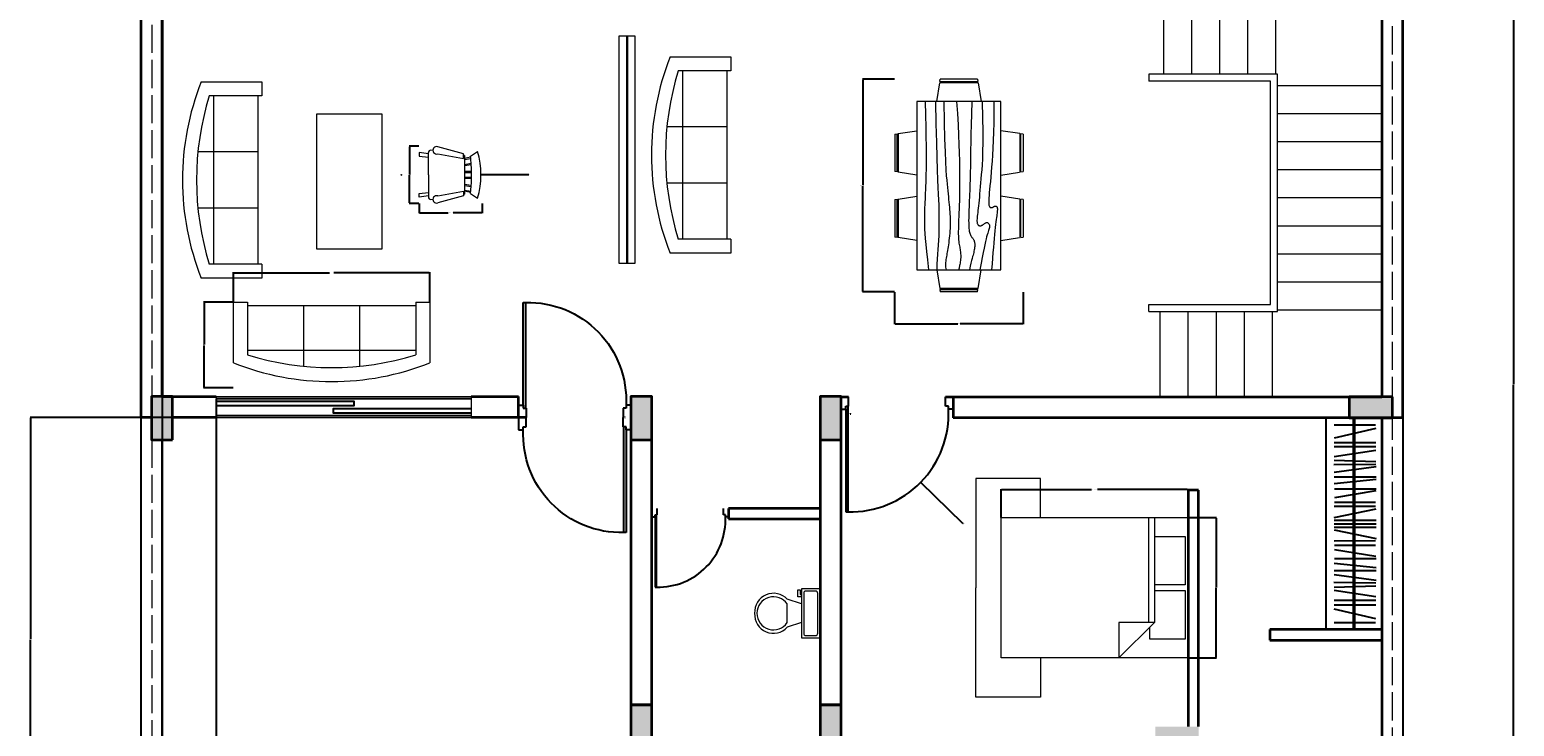
# Model space of a CAD drawing. Units: inches. Extents: x 2711 to 4246, y 540 to 1583.
# Tile 6 of 7: x 3610 to 4246, y 915 to 1213. Entities that reach past the tile are written whole.
import ezdxf

# ---------------------------------------------------------------- set-up
doc = ezdxf.new("R2010")
doc.units = ezdxf.units.IN
doc.linetypes.add('ACAD_ISO02W100', pattern=[15, 12, -3])
for name, color, linetype, lineweight in [('A-ANNO-DIMS', 2, 'Continuous', 18), ('A-COLS', 210, 'Continuous', 35), ('A-COLS-PATT', 6, 'Continuous', 13), ('A-FLOR-CASE', 30, 'Continuous', 18), ('A-FLOR-FIXT', 112, 'Continuous', 18), ('A-FLOR-STRS', 4, 'Continuous', 18), ('A-GLAZ', 4, 'Continuous', 18), ('A-WALL', 1, 'Continuous', 35), ('C-PROP-HIDN', 7, 'ACAD_ISO02W100', 13), ('C-PROP-WALL', 7, 'Continuous', 25), ('DOOR', 32, 'Continuous', 25), ('FURN', 30, 'Continuous', 18)]:
    doc.layers.add(name, color=color, linetype=linetype, lineweight=lineweight)
doc.layers.add('DARK', color=5, linetype='Continuous')
doc.layers.add('DECOR', color=30, linetype='Continuous')
doc.styles.get("Standard").update_dxf_attribs({"font": 'arial.ttf'})
doc.dimstyles.get("Standard").update_dxf_attribs({"dimtxt": 0.18, "dimasz": 0.18, "dimexe": 0.18, "dimexo": 0.0625, "dimgap": 0.09, "dimtad": 0, "dimtih": 1, "dimtoh": 1, "dimdec": 4, "dimzin": 0, "dimdsep": 46, "dimtxsty": 'Standard', "dimcen": 0.09, "dimadec": 0, "dimazin": 0, "dimtfac": 1, "dimtdec": 4, "dimtofl": 0, "dimtmove": 0, "dimatfit": 3, "dimfxl": 1, "dimtolj": 1, "dimtzin": 0, "dimarcsym": 0})

# ---------------------------------------------------------------- blocks, each defined once
blk = doc.blocks.new('DOORS')
at = {"layer": 'DOOR'}
for p, q in [((-0.63, -0.36), (-0.63, -5.61)), ((-0.63, -5.61), (1.37, -5.61)), ((1.37, -5.61), (1.37, -4.36)), ((1.37, -4.36), (2.62, -4.36)), ((1.37, -5.61), (1.37, -49.61)), ((2.37, -49.61), (2.37, -4.36)), ((2.62, -4.36), (2.62, -0.36)), ((44.12, -4.36), (44.12, -0.36)), ((45.37, -4.36), (44.12, -4.36)), ((47.37, -5.61), (45.37, -5.61)), ((47.37, -0.36), (47.37, -5.61)), ((1.37, -49.61), (2.37, -49.61))]:
    blk.add_line(p, q, dxfattribs=at)
for centre, radius, start, end in [((3.41, -7.61), 42.01, 268.5852, 2.73188), ((38.76, -4.99), 6.64, 354.60229, 5.39771)]:
    blk.add_arc(centre, radius, start, end, dxfattribs=at)
blk = doc.blocks.new('WARDROBE')
at = {"layer": 'DECOR'}
for p, q in [((24, 0), (0, 0)), ((0, 0), (0, -90.69)), ((11.75, 0), (11.75, -90.69)), ((11.78, 0), (11.78, -90.69)), ((11.8, 0), (11.8, -90.69)), ((11.83, 0), (11.83, -90.69)), ((11.85, 0), (11.85, -90.69)), ((11.88, 0), (11.88, -90.69)), ((11.92, 0), (11.92, -90.69)), ((11.95, 0), (11.95, -90.69)), ((11.97, 0), (11.97, -90.69)), ((12, 0), (12, -90.69)), ((12.03, 0), (12.03, -90.69)), ((12.06, 0), (12.06, -90.69)), ((12.1, 0), (12.1, -90.69)), ((12.14, 0), (12.14, -90.69)), ((12.17, 0), (12.17, -90.69)), ((12.2, 0), (12.2, -90.69)), ((12.22, 0), (12.22, -90.69)), ((12.25, 0), (12.25, -90.69)), ((12.25, 0), (12.25, -90.69)), ((24, -90.69), (24, 0)), ((3.53, -3.09), (21.27, -3.09)), ((21.48, -4.58), (3.53, -8.75)), ((3.53, -10.65), (21.48, -10.65)), ((21.48, -12.45), (3.53, -12.45)), ((21.48, -14.08), (3.53, -16.79)), ((3.53, -18.23), (21.48, -18.75)), ((21.48, -19.96), (3.47, -20.22)), ((21.49, -21.01), (3.52, -23.46)), ((3.52, -25.25), (21.49, -25.25)), ((21.49, -26.46), (3.52, -28.29)), ((3.74, -30.44), (21.49, -30.44)), ((21.36, -31.31), (3.74, -34.21)), ((21.29, -37.99), (3.52, -37.93)), ((3.74, -36.1), (21.29, -36.1)), ((3.52, -42.71), (21.49, -38.99)), ((3.52, -43.88), (21.49, -43.88)), ((3.52, -45.34), (21.49, -45.34)), ((3.52, -46.81), (21.49, -46.81)), ((3.52, -47.98), (21.49, -51.69)), ((21.29, -52.7), (3.52, -52.76)), ((3.74, -54.59), (21.29, -54.59)), ((21.36, -59.38), (3.74, -56.48)), ((21.49, -64.22), (3.52, -62.4)), ((3.74, -60.25), (21.49, -60.25)), ((3.52, -65.43), (21.49, -65.43)), ((21.49, -69.68), (3.52, -67.23)), ((21.48, -70.73), (3.47, -70.47)), ((3.53, -72.46), (21.48, -71.94)), ((21.48, -76.61), (3.53, -73.9)), ((21.48, -78.24), (3.53, -78.24)), ((3.53, -80.04), (21.48, -80.04)), ((21.48, -86.1), (3.53, -81.94)), ((3.53, -87.59), (21.27, -87.59)), ((0, -90.69), (24, -90.69))]:
    blk.add_line(p, q, dxfattribs=at)
blk = doc.blocks.new('DIPDASS')
at = {"layer": 'DARK'}
for p, q in [((0, 0), (109.02, 0)), ((0, -7.25), (109.02, -7.25))]:
    blk.add_line(p, q, dxfattribs=at)
at = {"layer": 'DOOR'}
for points in [[(0, -1.16), (56.28, -1.16), (58.81, -1.16), (58.81, -3.16), (56.28, -3.16), (0, -3.16)], [(109.02, -6.2), (52.74, -6.2), (50.21, -6.2), (50.21, -4.2), (52.74, -4.2), (109.02, -4.2)]]:
    blk.add_lwpolyline(points, dxfattribs=at)
blk = doc.blocks.new('Bed - Queen')
for p, q in [((0, -80.00003), (0, 0)), ((0, 0), (59.99999, 0)), ((59.99999, 0), (59.99999, -80.00003)), ((7.99999, -1.2), (28.79998, -1.2)), ((7.99999, -14.4), (7.99999, -1.2)), ((28.79998, -1.2), (28.79998, -14.4)), ((31.19999, -1.2), (51.99999, -1.2)), ((31.19999, -14.4), (31.19999, -1.2)), ((51.99999, -1.2), (51.99999, -16.4)), ((0, -14.4), (44.8, -14.4)), ((44.8, -16.8), (0, -16.8)), ((59.99999, -29.6), (44.8, -14.4)), ((44.8, -14.4), (44.8, -29.6)), ((51.99999, -16.4), (46.79936, -16.4)), ((44.8, -29.6), (59.99999, -29.6)), ((59.99999, -80.00003), (0, -80.00003))]:
    blk.add_line(p, q)
blk = doc.blocks.new('Dining Set - 36 x 72 in.')
for p, q in [((-22.2343, 26.00059), (-23.4847, 17.99762)), ((-22.2304, 26), (-5.7608, 26)), ((-22, 27.5), (-22.1562, 26.50042)), ((-5.8416, 26.5), (-22.1534, 26.5)), ((-22, 27.5), (-6, 27.5)), ((-5.8437, 26.49966), (-6, 27.5)), ((-4.5152, 17.99762), (-5.7655, 25.99926)), ((5.7657, 26.00059), (4.5153, 17.99762)), ((5.7696, 26), (22.2392, 26)), ((6, 27.5), (5.8438, 26.50042)), ((22.1584, 26.5), (5.8466, 26.5)), ((6, 27.5), (22, 27.5)), ((22.1563, 26.49966), (22, 27.5)), ((23.4848, 17.99762), (22.2345, 25.99926)), ((36, 18), (-36, 18)), ((-36, 18), (-36, -18)), ((36, -18), (36, 18)), ((-45.5, 8), (-44.5004, 8.15617)), ((-45.5, 8), (-45.5, -8)), ((-44.5, -8.15843), (-44.5, 8.15338)), ((-44.0006, 8.23428), (-35.9976, 9.48474)), ((-44, 8.23041), (-44, -8.23915)), ((44.0006, 8.23428), (35.9976, 9.48474)), ((44, 8.23041), (44, -8.23915)), ((44.5, -8.15843), (44.5, 8.15338)), ((45.5, 8), (44.5005, 8.15617)), ((45.5, 8), (45.5, -8)), ((-44.4997, -8.15631), (-45.5, -8)), ((-35.9976, -9.48476), (-43.9993, -8.2345)), ((35.9976, -9.48476), (43.9993, -8.2345)), ((44.4997, -8.15631), (45.5, -8)), ((-36, -18), (36, -18)), ((-22.2343, -26.0006), (-23.4847, -17.99762)), ((-4.5152, -17.99762), (-5.7655, -25.99928)), ((5.7657, -26.0006), (4.5153, -17.99762)), ((23.4848, -17.99762), (22.2345, -25.99928)), ((-22.2304, -26), (-5.7608, -26)), ((-22, -27.5), (-22.1562, -26.50044)), ((-5.8416, -26.5), (-22.1534, -26.5)), ((-22, -27.5), (-6, -27.5)), ((-5.8437, -26.49967), (-6, -27.5)), ((5.7696, -26), (22.2392, -26)), ((6, -27.5), (5.8438, -26.50044)), ((22.1584, -26.5), (5.8466, -26.5)), ((6, -27.5), (22, -27.5)), ((22.1563, -26.49967), (22, -27.5))]:
    blk.add_line(p, q)
for points in [[(-36, 15), (-31.1772, 14.97754), (-26.8079, 14.91406), (-22.8538, 14.81543), (-19.276, 14.6875), (-16.0362, 14.53613), (-13.0957, 14.36718), (-10.4159, 14.18652), (-7.9583, 14), (-5.6904, 13.81315), (-3.6035, 13.63021), (-1.6954, 13.45508), (0.0365, 13.29166), (1.5945, 13.14388), (2.9811, 13.01562), (4.1988, 12.9108), (5.25, 12.83333), (6.1393, 12.78613), (6.8802, 12.76823), (7.4883, 12.77767), (7.9792, 12.8125), (8.3685, 12.87077), (8.6719, 12.95052), (8.9049, 13.0498), (9.0833, 13.16666), (9.2205, 13.29899), (9.3216, 13.44401), (9.3895, 13.59879), (9.4271, 13.76041), (9.4373, 13.92594), (9.4232, 14.09245), (9.3875, 14.257), (9.3333, 14.41666), (9.2638, 14.56917), (9.1836, 14.71484), (9.0975, 14.85465), (9.0104, 14.98958), (8.9272, 15.1206), (8.8529, 15.2487), (8.7922, 15.37483), (8.75, 15.5), (8.7305, 15.62467), (8.7344, 15.74739), (8.7617, 15.86621), (8.8125, 15.97916), (8.8867, 16.08431), (8.9844, 16.17968), (9.1055, 16.26334), (9.25, 16.33333), (9.4189, 16.38802), (9.6172, 16.42708), (9.8506, 16.45052), (10.125, 16.45833), (10.4463, 16.45052), (10.8203, 16.42708), (11.2529, 16.38802), (11.75, 16.33333), (12.3184, 16.26318), (12.9694, 16.17838), (13.7151, 16.07991), (14.5677, 15.96875), (15.5395, 15.84586), (16.6426, 15.71224), (17.8893, 15.56884), (19.2917, 15.41666), (20.859, 15.25667), (22.5879, 15.08984), (24.4721, 14.91715), (26.5052, 14.73958), (28.6809, 14.5581), (30.9929, 14.3737), (33.4347, 14.18733), (36, 14)], [(-36, 10), (-28.9766, 10.14274), (-23.1725, 10.20442), (-18.4241, 10.19775), (-14.5677, 10.13541), (-11.4399, 10.03011), (-8.877, 9.89453), (-6.7154, 9.74137), (-4.7917, 9.58333), (-2.9698, 9.43082), (-1.2246, 9.28515), (0.4415, 9.14534), (2.026, 9.01041), (3.5266, 8.87939), (4.9408, 8.7513), (6.266, 8.62516), (7.5, 8.5), (8.6411, 8.37549), (9.6914, 8.2539), (10.6538, 8.13818), (11.5312, 8.03125), (12.3267, 7.93603), (13.043, 7.85547), (13.6831, 7.79248), (14.25, 7.75), (14.7471, 7.7303), (15.1797, 7.73307), (15.5537, 7.75732), (15.875, 7.80208), (16.1494, 7.86637), (16.3828, 7.94922), (16.5811, 8.04964), (16.75, 8.16666), (16.8944, 8.29915), (17.0143, 8.44531), (17.1089, 8.60319), (17.1771, 8.77083), (17.218, 8.94629), (17.2305, 9.1276), (17.2137, 9.31282), (17.1667, 9.5), (17.0895, 9.6875), (16.987, 9.875), (16.8649, 10.0625), (16.7292, 10.25), (16.5856, 10.4375), (16.4401, 10.625), (16.2985, 10.8125), (16.1667, 11), (16.05, 11.18733), (15.9518, 11.3737), (15.8752, 11.5581), (15.8229, 11.73958), (15.798, 11.91715), (15.8034, 12.08984), (15.842, 12.25667), (15.9167, 12.41666), (16.0295, 12.56836), (16.1784, 12.70833), (16.3605, 12.83268), (16.5729, 12.9375), (16.8127, 13.01888), (17.0768, 13.07291), (17.3625, 13.0957), (17.6667, 13.08333), (17.9894, 13.03312), (18.3418, 12.94726), (18.7382, 12.82918), (19.1927, 12.68229), (19.7195, 12.51001), (20.3327, 12.31575), (21.0465, 12.10294), (21.875, 11.875), (22.8357, 11.63354), (23.959, 11.37304), (25.2786, 11.08618), (26.8282, 10.76562), (28.6414, 10.40405), (30.752, 9.99414), (33.1936, 9.52856), (36, 9)], [(-36, 5.5), (-30.7157, 5.3348), (-26.069, 5.20963), (-21.9946, 5.11767), (-18.4271, 5.05208), (-15.3009, 5.00602), (-12.5508, 4.97265), (-10.1112, 4.94515), (-7.9167, 4.91666), (-5.909, 4.88167), (-4.0586, 4.83984), (-2.3429, 4.79215), (-0.7396, 4.73958), (0.7739, 4.6831), (2.22, 4.6237), (3.6213, 4.56233), (5, 4.5), (6.373, 4.43782), (7.7344, 4.3776), (9.0723, 4.32129), (10.375, 4.27083), (11.6309, 4.22819), (12.8281, 4.19531), (13.9551, 4.17415), (15, 4.16666), (15.954, 4.17448), (16.819, 4.19791), (17.6001, 4.23698), (18.3021, 4.29166), (18.9299, 4.36198), (19.4883, 4.44791), (19.9823, 4.54948), (20.4167, 4.66666), (20.7969, 4.79899), (21.1302, 4.94401), (21.4245, 5.09879), (21.6875, 5.26041), (21.9271, 5.42594), (22.1511, 5.59245), (22.3672, 5.757), (22.5834, 5.91666), (22.8065, 6.06868), (23.0404, 6.21093), (23.2879, 6.34147), (23.5521, 6.45833), (23.8358, 6.55957), (24.142, 6.64323), (24.4735, 6.70735), (24.8334, 6.75), (25.2235, 6.76969), (25.642, 6.76692), (26.0858, 6.74267), (26.5521, 6.69791), (27.0379, 6.63362), (27.5404, 6.55078), (28.0565, 6.45036), (28.5834, 6.33333), (29.1242, 6.19987), (29.7071, 6.04687), (30.3661, 5.87044), (31.1354, 5.66666), (32.0493, 5.43164), (33.142, 5.16146), (34.4475, 4.85221), (36, 4.5)], [(-36, -1), (-30.7915, -0.6591), (-26.0195, -0.38216), (-21.6519, -0.16284), (-17.6563, 0.00521), (-14.0005, 0.12833), (-10.6523, 0.21289), (-7.5796, 0.26522), (-4.75, 0.29166), (-2.134, 0.29793), (0.2878, 0.28711), (2.5317, 0.26163), (4.6146, 0.22396), (6.5529, 0.17651), (8.3633, 0.12174), (10.0623, 0.06209), (11.6667, 0), (13.1899, -0.06201), (14.6341, -0.1211), (15.9982, -0.17432), (17.2813, -0.21875), (18.4823, -0.25147), (19.6003, -0.26953), (20.6343, -0.27002), (21.5834, -0.25), (22.4481, -0.20768), (23.2357, -0.14584), (23.9549, -0.06836), (24.6146, 0.02083), (25.2235, 0.11784), (25.7904, 0.21875), (26.3241, 0.31966), (26.8334, 0.41666), (27.3265, 0.50618), (27.8099, 0.58593), (28.2894, 0.65397), (28.7709, 0.70833), (29.2601, 0.74707), (29.763, 0.76823), (30.2855, 0.76985), (30.8334, 0.75), (31.4088, 0.70784), (31.9994, 0.64713), (32.589, 0.57275), (33.1615, 0.48958), (33.7008, 0.4025), (34.1908, 0.3164), (34.6153, 0.23616), (34.9584, 0.16666), (35.2099, 0.11165), (35.3848, 0.07031), (35.504, 0.04069), (35.5886, 0.02083), (35.6594, 0.00879), (35.7377, 0.0026), (35.8442, 0.00032), (36, 0)], [(-36, -6.5), (-27.1843, -6.31267), (-20.084, -6.1263), (-14.469, -5.9419), (-10.1094, -5.76042), (-6.7752, -5.58285), (-4.2363, -5.41016), (-2.2629, -5.24333), (-0.625, -5.08334), (0.8708, -4.93099), (2.2715, -4.78646), (3.5872, -4.64974), (4.8281, -4.52084), (6.0046, -4.39974), (7.127, -4.28646), (8.2053, -4.18099), (9.25, -4.08334), (10.2705, -3.99382), (11.2734, -3.91407), (12.2647, -3.84603), (13.25, -3.79167), (14.2354, -3.75293), (15.2266, -3.73177), (16.2295, -3.73015), (17.25, -3.75), (18.2912, -3.79248), (19.3451, -3.85547), (20.4009, -3.93604), (21.4479, -4.03125), (22.4754, -4.13819), (23.4727, -4.25391), (24.4289, -4.37549), (25.3334, -4.5), (26.1785, -4.62492), (26.9694, -4.74935), (27.7145, -4.87281), (28.4219, -4.99479), (29.1, -5.11483), (29.7572, -5.23242), (30.4016, -5.34709), (31.0417, -5.45834), (31.6837, -5.56437), (32.3262, -5.65821), (32.9658, -5.73153), (33.599, -5.77604), (34.2224, -5.78345), (34.8327, -5.74545), (35.4264, -5.65373), (36, -5.5)], [(-36, -10), (-26.4022, -9.81299), (-18.4675, -9.62891), (-11.9839, -9.45069), (-6.7396, -9.28125), (-2.5226, -9.12354), (0.8789, -8.98047), (3.6769, -8.85498), (6.0833, -8.75), (8.2767, -8.66765), (10.3021, -8.60677), (12.1712, -8.56543), (13.8958, -8.54167), (15.4876, -8.53353), (16.9583, -8.53907), (18.3197, -8.55632), (19.5834, -8.58334), (20.7616, -8.61841), (21.8685, -8.66081), (22.9188, -8.71004), (23.9271, -8.76563), (24.9081, -8.82707), (25.8763, -8.89388), (26.8465, -8.96558), (27.8334, -9.04167), (28.8474, -9.12118), (29.8828, -9.20117), (30.93, -9.27824), (31.9792, -9.34896), (33.0205, -9.40991), (34.0443, -9.45768), (35.0407, -9.48885), (36, -9.5)], [(-36, -14.5), (-30.0881, -14.33513), (-25.0332, -14.21224), (-20.7312, -14.12647), (-17.0781, -14.07292), (-13.97, -14.04671), (-11.3027, -14.04297), (-8.9724, -14.05681), (-6.875, -14.08334), (-4.9224, -14.11833), (-3.0905, -14.16016), (-1.3709, -14.20785), (0.2448, -14.26042), (1.7647, -14.3169), (3.1973, -14.3763), (4.5507, -14.43767), (5.8333, -14.5), (7.0554, -14.5621), (8.235, -14.62175), (9.3922, -14.67652), (10.5469, -14.72396), (11.7192, -14.76164), (12.929, -14.78711), (14.1965, -14.79794), (15.5417, -14.79167), (16.9933, -14.76424), (18.6152, -14.70508), (20.4804, -14.60197), (22.6615, -14.44271), (25.2312, -14.21509), (28.2624, -13.9069), (31.8277, -13.50594), (36, -13)]]:
    blk.add_lwpolyline(points)
blk = doc.blocks.new('Sofa - Roundback 7 ft.')
for p, q in [((-36.000027, -34), (-36.000027, -11.4696)), ((-12.00002, -32.4421), (-12.00003, -6.5971)), ((11.99997, -32.4421), (11.99998, -6.5971)), ((35.99998, -34), (35.99998, -11.4696)), ((-35.999844, -13.3819), (35.9998, -13.3819)), ((-36.000027, -32.4421), (35.99998, -32.4421))]:
    blk.add_line(p, q)
for points in [[(-36.000027, -34), (-42.000027, -34), (-42.000027, -8)], [(41.99998, -8), (41.99998, -34), (35.99998, -34)]]:
    blk.add_lwpolyline(points)
for centre, radius, start, end in [((0, -114.25), 114.25, 68.43141, 111.5686), ((-0.00001, -127.1968), 121.1968, 72.72033, 107.2797)]:
    blk.add_arc(centre, radius, start, end)
blk = doc.blocks.new('Chair - Rocking')
for p, q in [((-8, -4.5), (-10, -1.5)), ((-7.5, -4.5), (-7, -7)), ((-6.5, -7), (-7.02225, -4.43)), ((-4.5, -7), (-4.96674, -4.19951)), ((-4, -7), (-4.40532, -4.16272)), ((-1.5, -4.05012), (-1.5, -7)), ((-1, -7), (-1, -4.05012)), ((1, -7), (1, -4.04655)), ((1.5, -4.05012), (1.5, -7)), ((4, -7), (4.40187, -4.18694)), ((4.5, -7), (4.96761, -4.19437)), ((6.5, -7), (7, -4.4057)), ((7.5, -4.5), (7, -7)), ((8, -4.5), (10, -1.5)), ((-9, -7.5), (-12, -18.49999)), ((-7, -7.5), (-9, -7.5)), ((-9, -18.49999), (-7, -7.5)), ((-8.23428, -6.99939), (-8.3093, -7.47958)), ((-8.23041, -7), (8.23915, -7)), ((7, -7.5), (9, -7.5)), ((9, -18.49999), (7, -7.5)), ((8.31071, -7.48854), (8.23449, -7.00073)), ((9, -7.5), (12, -18.49999)), ((-10.36644, -20.64523), (-10.5, -21.49999)), ((-9, -22.49999), (-9.5, -26.49999)), ((0, -22.49999), (-9.5, -22.49999)), ((-8, -26.49999), (-7.5, -22.49999)), ((0, -22.49999), (9.5, -22.49999)), ((8, -26.49999), (7.5, -22.49999)), ((9, -22.49999), (9.5, -26.49999)), ((10.5, -21.49999), (10.3575, -20.58798)), ((-9.5, -26.49999), (-8, -26.49999)), ((9.5, -26.49999), (8, -26.49999))]:
    blk.add_line(p, q)
for centre, radius, start, end in [((0, -34.08333), 34.08333, 72.93847, 107.0615), ((0, -68.25004), 64.25, 93.92211, 97.15267), ((0, -68.25004), 64.25, 82.84733, 93.92211), ((-10.5, -18.99999), 1.58114, 161.5651, 18.43495), ((10.5, -18.99999), 1.58114, 161.5651, 18.43495), ((-9.5, -21.49999), 1, 180, 270), ((9.5, -21.49999), 1, 270, 0)]:
    blk.add_arc(centre, radius, start, end)
blk = doc.blocks.new('*U44')
for p, q in [((9.5, -6), (9.5, -2)), ((-10, -8.5), (-8, -8.5)), ((-10, -9.5), (-10, -8.5)), ((-7, -9.5), (-10, -9.5)), ((-8, -8.5), (-8, -8)), ((-7, -8), (-7, -9.5)), ((-4, -8), (-6, -14)), ((4, -8), (6, -14)), ((4, -14), (-4, -14))]:
    blk.add_line(p, q)
blk.add_lwpolyline([(10.5, -8), (10.5, 0), (-10.5, 0), (-10.5, -8)], close=True)
for points in [[(-9.5, -2), (-9.5, -6)], [(8.5, -1), (-8.5, -1)], [(-8.5, -7), (8.5, -7)]]:
    blk.add_lwpolyline(points)
for centre, radius, start, end in [((-8.625, -1.875), 0.8839, 81.8699, 188.1301), ((-8.625, -6.125), 0.8839, 171.869898, 278.1301), ((8.625, -1.875), 0.8839, 351.8699, 98.1301), ((8.625, -6.125), 0.8839, 261.8699, 8.1301), ((-0.4772, -19.9188), 8.0953, 133.01722, 273.38), ((0.0374, -19.8731), 7.127, 124.50543, 269.7), ((-0.0373, -19.8731), 7.127, 270.3, 55.4946), ((0.4773, -19.9188), 8.0953, 266.62, 46.9828)]:
    blk.add_arc(centre, radius, start, end)
blk = doc.blocks.new('STAIR-RETURN')
for p, q in [((6.2, 174.01), (6.2, 138.01)), ((18.2, 174.01), (18.2, 138.01)), ((30.2, 174.01), (30.2, 138.01)), ((42.2, 174.01), (42.2, 138.01)), ((54.2, 174.01), (54.2, 138.01)), ((55.04, 138.01), (0, 138.01)), ((0, 138.01), (0, 135.01)), ((52.04, 135.01), (0, 135.01)), ((52.04, 39.5), (52.04, 135.01)), ((55.04, 133.05), (55.04, 138.01)), ((99.72, 133.05), (55.04, 133.05)), ((55.04, 37.05), (55.04, 133.05)), ((99.72, 121.05), (55.04, 121.05)), ((99.72, 109.05), (55.04, 109.05)), ((99.72, 97.05), (55.04, 97.05)), ((99.72, 85.05), (55.04, 85.05)), ((99.72, 73.05), (55.04, 73.05)), ((99.72, 61.05), (55.04, 61.05)), ((99.72, 49.05), (55.04, 49.05)), ((0, 36.5), (0, 39.5)), ((0, 39.5), (52.04, 39.5)), ((0, 36.5), (52.73, 36.5)), ((4.73, 36.5), (4.74, 0)), ((16.73, 36.5), (16.74, 0)), ((28.73, 36.5), (28.74, 0)), ((40.73, 36.5), (40.74, 0)), ((52.73, 36.5), (52.74, 0)), ((52.73, 36.5), (55.04, 36.5)), ((99.72, 37.05), (55.04, 37.05)), ((55.04, 36.5), (55.04, 37.05))]:
    blk.add_line(p, q)
blk = doc.blocks.new('SCREEN-LIVING')
for p, q in [((0, 97.11), (0, 0)), ((7, 97.11), (0, 97.11)), ((3.25, 97.11), (3.25, 0)), ((3.5, 97.11), (3.5, 0)), ((3.75, 97.11), (3.75, 0)), ((7, 0), (7, 97.11)), ((0, 0), (7, 0))]:
    blk.add_line(p, q)
blk = doc.blocks.new('BED-BASE-QUEEN')
for p, q in [((27.64, 93.59), (0, 93.59)), ((0, 93.59), (0, 46.79)), ((27.64, 76.79), (27.64, 93.59)), ((0, 0), (0, 46.79)), ((27.64, 16.79), (27.64, 0)), ((27.64, 0), (0, 0))]:
    blk.add_line(p, q)
blk = doc.blocks.new('*D60')
at = {"layer": 'A-ANNO-DIMS', "color": 0, "lineweight": -2, "transparency": 16777216}
for p, q in [((3697.65, 1096.46), (3697.65, 1109.18)), ((3697.83, 1109), (3738.74, 1109)), ((3781.47, 1109), (3740.55, 1109)), ((3781.65, 1096.46), (3781.65, 1109.18))]:
    blk.add_line(p, q, dxfattribs=at)
at = {"layer": 'A-ANNO-DIMS', "color": 0, "transparency": 16777216}
for points in [[(3697.83, 1109.03), (3697.83, 1108.97), (3697.65, 1109)], [(3781.47, 1109.03), (3781.47, 1108.97), (3781.65, 1109)]]:
    blk.add_solid(points, dxfattribs=at)
at = {"layer": 'Defpoints', "color": 0, "transparency": 16777216}
for p in [(3697.65, 1109), (3697.65, 1096.4), (3781.65, 1096.4)]:
    blk.add_point(p, dxfattribs=at)
at = {"layer": 'A-ANNO-DIMS', "color": 0, "transparency": 16777216, "insert": (3739.65, 1109), "char_height": 0.18, "attachment_point": 5}
blk.add_mtext('\\A1;SOFA 84 TYP.', dxfattribs=at)
blk = doc.blocks.new('*D61')
at = {"layer": 'A-ANNO-DIMS', "color": 0, "lineweight": -2, "transparency": 16777216}
for p, q in [((3697.58, 1096.4), (3684.87, 1096.4)), ((3685.05, 1096.22), (3685.05, 1078.25)), ((3685.05, 1059.91), (3685.05, 1077.89)), ((3697.58, 1059.73), (3684.87, 1059.73))]:
    blk.add_line(p, q, dxfattribs=at)
at = {"layer": 'A-ANNO-DIMS', "color": 0, "transparency": 16777216}
for points in [[(3685.02, 1096.22), (3685.08, 1096.22), (3685.05, 1096.4)], [(3685.02, 1059.91), (3685.08, 1059.91), (3685.05, 1059.73)]]:
    blk.add_solid(points, dxfattribs=at)
at = {"layer": 'Defpoints', "color": 0, "transparency": 16777216}
for p in [(3697.65, 1096.4), (3685.05, 1059.73), (3697.65, 1059.73)]:
    blk.add_point(p, dxfattribs=at)
at = {"layer": 'A-ANNO-DIMS', "color": 0, "transparency": 16777216, "insert": (3685.05, 1078.07), "char_height": 0.18, "attachment_point": 5}
blk.add_mtext('\\A1;37 TYP.', dxfattribs=at)
blk = doc.blocks.new('*D70')
at = {"layer": 'A-ANNO-DIMS', "color": 0, "lineweight": -2, "transparency": 16777216}
for p, q in [((4026.21, 1004.25), (4026.21, 1016.37)), ((4026.39, 1016.19), (4064.9, 1016.19)), ((4106.03, 1016.19), (4067.51, 1016.19)), ((4106.21, 1004.25), (4106.21, 1016.37))]:
    blk.add_line(p, q, dxfattribs=at)
at = {"layer": 'A-ANNO-DIMS', "color": 0, "transparency": 16777216}
for points in [[(4026.39, 1016.22), (4026.39, 1016.16), (4026.21, 1016.19)], [(4106.03, 1016.22), (4106.03, 1016.16), (4106.21, 1016.19)]]:
    blk.add_solid(points, dxfattribs=at)
at = {"layer": 'Defpoints', "color": 0, "transparency": 16777216}
for p in [(4106.21, 1016.19), (4026.21, 1004.19), (4106.21, 1004.19)]:
    blk.add_point(p, dxfattribs=at)
at = {"layer": 'A-ANNO-DIMS', "color": 0, "transparency": 16777216, "insert": (4066.21, 1016.19), "char_height": 0.18, "attachment_point": 5}
blk.add_mtext('\\A1;QUEEN BED 80 TYP.', dxfattribs=at)
blk = doc.blocks.new('*D71')
at = {"layer": 'A-ANNO-DIMS', "color": 0, "lineweight": -2, "transparency": 16777216}
for p, q in [((4106.27, 1004.19), (4118.39, 1004.19)), ((4118.21, 1004.01), (4118.21, 974.37)), ((4118.21, 944.37), (4118.21, 974)), ((4106.27, 944.19), (4118.39, 944.19))]:
    blk.add_line(p, q, dxfattribs=at)
at = {"layer": 'A-ANNO-DIMS', "color": 0, "transparency": 16777216}
for points in [[(4118.18, 1004.01), (4118.24, 1004.01), (4118.21, 1004.19)], [(4118.18, 944.37), (4118.24, 944.37), (4118.21, 944.19)]]:
    blk.add_solid(points, dxfattribs=at)
at = {"layer": 'Defpoints', "color": 0, "transparency": 16777216}
for p in [(4106.21, 1004.19), (4106.21, 944.19), (4118.21, 944.19)]:
    blk.add_point(p, dxfattribs=at)
at = {"layer": 'A-ANNO-DIMS', "color": 0, "transparency": 16777216, "insert": (4118.21, 974.19), "char_height": 0.18, "attachment_point": 5}
blk.add_mtext('\\A1;60 TYP.', dxfattribs=at)
blk = doc.blocks.new('*D76')
at = {"layer": 'A-ANNO-DIMS', "color": 0, "lineweight": -2, "transparency": 16777216}
for p, q in [((3980.59, 1191.78), (3966.82, 1191.78)), ((3967, 1191.6), (3967, 1146.46)), ((3967, 1100.96), (3967, 1146.1)), ((3980.59, 1100.78), (3966.82, 1100.78))]:
    blk.add_line(p, q, dxfattribs=at)
at = {"layer": 'A-ANNO-DIMS', "color": 0, "transparency": 16777216}
for points in [[(3966.97, 1191.6), (3967.03, 1191.6), (3967, 1191.78)], [(3966.97, 1100.96), (3967.03, 1100.96), (3967, 1100.78)]]:
    blk.add_solid(points, dxfattribs=at)
at = {"layer": 'Defpoints', "color": 0, "transparency": 16777216}
for p in [(3980.65, 1191.78), (3967, 1100.78), (3980.65, 1100.78)]:
    blk.add_point(p, dxfattribs=at)
at = {"layer": 'A-ANNO-DIMS', "color": 0, "transparency": 16777216, "insert": (3967, 1146.28), "char_height": 0.18, "attachment_point": 5}
blk.add_mtext('\\A1;DINING SET 91 TYP.', dxfattribs=at)
blk = doc.blocks.new('*D77')
at = {"layer": 'A-ANNO-DIMS', "color": 0, "lineweight": -2, "transparency": 16777216}
for p, q in [((3980.65, 1100.72), (3980.65, 1086.95)), ((4035.65, 1100.72), (4035.65, 1086.95)), ((3980.83, 1087.13), (4007.62, 1087.13)), ((4035.47, 1087.13), (4008.68, 1087.13))]:
    blk.add_line(p, q, dxfattribs=at)
at = {"layer": 'A-ANNO-DIMS', "color": 0, "transparency": 16777216}
for points in [[(3980.83, 1087.16), (3980.83, 1087.1), (3980.65, 1087.13)], [(4035.47, 1087.16), (4035.47, 1087.1), (4035.65, 1087.13)]]:
    blk.add_solid(points, dxfattribs=at)
at = {"layer": 'Defpoints', "color": 0, "transparency": 16777216}
for p in [(3980.65, 1100.78), (4035.65, 1100.78), (4035.65, 1087.13)]:
    blk.add_point(p, dxfattribs=at)
at = {"layer": 'A-ANNO-DIMS', "color": 0, "transparency": 16777216, "insert": (4008.15, 1087.13), "char_height": 0.18, "attachment_point": 5}
blk.add_mtext('\\A1;55 TYP.', dxfattribs=at)
blk = doc.blocks.new('*D78')
at = {"layer": 'A-ANNO-DIMS', "color": 0, "lineweight": -2, "transparency": 16777216}
for p, q in [((3777.09, 1138.6), (3777.09, 1134.44)), ((3804.09, 1138.6), (3804.09, 1134.44)), ((3777.27, 1134.62), (3789.49, 1134.62)), ((3803.91, 1134.62), (3791.68, 1134.62))]:
    blk.add_line(p, q, dxfattribs=at)
at = {"layer": 'A-ANNO-DIMS', "color": 0, "transparency": 16777216}
for points in [[(3777.27, 1134.65), (3777.27, 1134.59), (3777.09, 1134.62)], [(3803.91, 1134.65), (3803.91, 1134.59), (3804.09, 1134.62)]]:
    blk.add_solid(points, dxfattribs=at)
at = {"layer": 'Defpoints', "color": 0, "transparency": 16777216}
for p in [(3777.09, 1138.67), (3804.09, 1138.67), (3804.09, 1134.62)]:
    blk.add_point(p, dxfattribs=at)
at = {"layer": 'A-ANNO-DIMS', "color": 0, "transparency": 16777216, "insert": (3790.59, 1134.62), "char_height": 0.18, "attachment_point": 5}
blk.add_mtext('\\A1;ROCKER 27 TYP.', dxfattribs=at)
blk = doc.blocks.new('*D79')
at = {"layer": 'A-ANNO-DIMS', "color": 0, "lineweight": -2, "transparency": 16777216}
for p, q in [((3777.02, 1163.1), (3772.86, 1163.1)), ((3773.04, 1162.92), (3773.04, 1151.06)), ((3773.04, 1138.85), (3773.04, 1150.7)), ((3777.02, 1138.67), (3772.86, 1138.67))]:
    blk.add_line(p, q, dxfattribs=at)
at = {"layer": 'A-ANNO-DIMS', "color": 0, "transparency": 16777216}
for points in [[(3773.01, 1162.92), (3773.07, 1162.92), (3773.04, 1163.1)], [(3773.01, 1138.85), (3773.07, 1138.85), (3773.04, 1138.67)]]:
    blk.add_solid(points, dxfattribs=at)
at = {"layer": 'Defpoints', "color": 0, "transparency": 16777216}
for p in [(3777.09, 1163.1), (3773.04, 1138.67), (3777.09, 1138.67)]:
    blk.add_point(p, dxfattribs=at)
at = {"layer": 'A-ANNO-DIMS', "color": 0, "transparency": 16777216, "insert": (3773.04, 1150.88), "char_height": 0.18, "attachment_point": 5}
blk.add_mtext('\\A1;24 TYP.', dxfattribs=at)
blk = doc.blocks.new('*D97')
at = {"layer": 'A-ANNO-DIMS', "color": 0, "lineweight": -2, "transparency": 16777216}
for p, q in [((4198.24, 1534.95), (4245.74, 1534.95)), ((4245.56, 1534.77), (4245.56, 1061.38)), ((4245.56, 587.63), (4245.56, 1061.02)), ((4198.24, 587.45), (4245.74, 587.45))]:
    blk.add_line(p, q, dxfattribs=at)
at = {"layer": 'A-ANNO-DIMS', "color": 0, "transparency": 16777216}
for points in [[(4245.53, 1534.77), (4245.59, 1534.77), (4245.56, 1534.95)], [(4245.53, 587.63), (4245.59, 587.63), (4245.56, 587.45)]]:
    blk.add_solid(points, dxfattribs=at)
at = {"layer": 'Defpoints', "color": 0, "transparency": 16777216}
for p in [(4198.18, 1534.95), (4245.56, 1534.95), (4198.18, 587.45)]:
    blk.add_point(p, dxfattribs=at)
at = {"layer": 'A-ANNO-DIMS', "color": 0, "transparency": 16777216, "insert": (4245.56, 1061.2), "char_height": 0.18, "attachment_point": 5}
blk.add_mtext('\\A1;947.5', dxfattribs=at)
blk = doc.blocks.new('*D105')
at = {"layer": 'A-ANNO-DIMS', "color": 0, "lineweight": -2, "transparency": 16777216}
for p, q in [((3667.18, 1055.98), (3667.18, 539.89)), ((3690.29, 1055.1), (3690.29, 539.89)), ((3667.36, 540.07), (3678.36, 540.07)), ((3690.11, 540.07), (3679.12, 540.07))]:
    blk.add_line(p, q, dxfattribs=at)
at = {"layer": 'A-ANNO-DIMS', "color": 0, "transparency": 16777216}
for points in [[(3667.36, 540.1), (3667.36, 540.04), (3667.18, 540.07)], [(3690.11, 540.1), (3690.11, 540.04), (3690.29, 540.07)]]:
    blk.add_solid(points, dxfattribs=at)
at = {"layer": 'Defpoints', "color": 0, "transparency": 16777216}
for p in [(3667.18, 1056.04), (3690.29, 1055.17), (3690.29, 540.07)]:
    blk.add_point(p, dxfattribs=at)
at = {"layer": 'A-ANNO-DIMS', "color": 0, "transparency": 16777216, "insert": (3678.74, 540.07), "char_height": 0.18, "attachment_point": 5}
blk.add_mtext('\\A1;23.11', dxfattribs=at)
blk = doc.blocks.new('*D106')
at = {"layer": 'A-ANNO-DIMS', "color": 0, "lineweight": -2, "transparency": 16777216}
for p, q in [((3690.29, 1055.1), (3690.29, 539.89)), ((3867.71, 1046.98), (3867.71, 539.89)), ((3690.47, 540.07), (3778.62, 540.07)), ((3867.53, 540.07), (3779.39, 540.07))]:
    blk.add_line(p, q, dxfattribs=at)
at = {"layer": 'A-ANNO-DIMS', "color": 0, "transparency": 16777216}
for points in [[(3690.47, 540.1), (3690.47, 540.04), (3690.29, 540.07)], [(3867.53, 540.1), (3867.53, 540.04), (3867.71, 540.07)]]:
    blk.add_solid(points, dxfattribs=at)
at = {"layer": 'Defpoints', "color": 0, "transparency": 16777216}
for p in [(3690.29, 1055.17), (3867.71, 1047.04), (3867.71, 540.07)]:
    blk.add_point(p, dxfattribs=at)
at = {"layer": 'A-ANNO-DIMS', "color": 0, "transparency": 16777216, "insert": (3779, 540.07), "char_height": 0.18, "attachment_point": 5}
blk.add_mtext('\\A1;177.4', dxfattribs=at)
blk = doc.blocks.new('*D125')
at = {"layer": 'A-ANNO-DIMS', "color": 0, "lineweight": -2, "transparency": 16777216}
for p, q in [((3671.47, 1047.04), (3610.62, 1047.04)), ((3610.8, 1046.86), (3610.8, 952.14)), ((3610.8, 857.05), (3610.8, 951.78)), ((3666.97, 856.87), (3610.62, 856.87))]:
    blk.add_line(p, q, dxfattribs=at)
at = {"layer": 'A-ANNO-DIMS', "color": 0, "transparency": 16777216}
for points in [[(3610.77, 1046.86), (3610.83, 1046.86), (3610.8, 1047.04)], [(3610.77, 857.05), (3610.83, 857.05), (3610.8, 856.87)]]:
    blk.add_solid(points, dxfattribs=at)
at = {"layer": 'Defpoints', "color": 0, "transparency": 16777216}
for p in [(3610.8, 1047.04), (3671.53, 1047.04), (3667.03, 856.87)]:
    blk.add_point(p, dxfattribs=at)
at = {"layer": 'A-ANNO-DIMS', "color": 0, "transparency": 16777216, "insert": (3610.8, 951.96), "char_height": 0.18, "attachment_point": 5}
blk.add_mtext('\\A1;190.16', dxfattribs=at)
blk = doc.blocks.new('*D129')
at = {"layer": 'A-ANNO-DIMS', "color": 0, "lineweight": -2, "transparency": 16777216}
for p, q in [((3961.65, 1048.67), (3961.83, 1048.67)), ((3961.74, 1048.58), (3961.74, 1048.76)), ((4009.82, 1001.69), (3991.92, 1019.18)), ((4010, 1001.69), (4009.82, 1001.69))]:
    blk.add_line(p, q, dxfattribs=at)
at = {"layer": 'A-ANNO-DIMS', "color": 0, "transparency": 16777216}
blk.add_solid([(3991.94, 1019.2), (3991.9, 1019.16), (3991.79, 1019.31)], dxfattribs=at)
at = {"layer": 'Defpoints', "color": 0, "transparency": 16777216}
for p in [(3961.74, 1048.67), (3991.79, 1019.31)]:
    blk.add_point(p, dxfattribs=at)
at = {"layer": 'A-ANNO-DIMS', "color": 0, "transparency": 16777216, "insert": (4010.46, 1001.69), "char_height": 0.18, "attachment_point": 5}
blk.add_mtext('\\A1;R42.01', dxfattribs=at)
blk = doc.blocks.new('*D130')
at = {"layer": 'A-ANNO-DIMS', "color": 0, "lineweight": -2, "transparency": 16777216}
for p, q in [((3769.41, 1150.88), (3769.59, 1150.88)), ((3769.5, 1150.79), (3769.5, 1150.97)), ((3824.04, 1150.88), (3803.77, 1150.88))]:
    blk.add_line(p, q, dxfattribs=at)
at = {"layer": 'A-ANNO-DIMS', "color": 0, "transparency": 16777216}
blk.add_solid([(3803.77, 1150.91), (3803.77, 1150.85), (3803.59, 1150.88)], dxfattribs=at)
at = {"layer": 'Defpoints', "color": 0, "transparency": 16777216}
for p in [(3769.5, 1150.88), (3803.59, 1150.88)]:
    blk.add_point(p, dxfattribs=at)
at = {"layer": 'A-ANNO-DIMS', "color": 0, "transparency": 16777216, "insert": (3824.52, 1150.88), "char_height": 0.18, "attachment_point": 5}
blk.add_mtext('\\A1;R34.08', dxfattribs=at)

msp = doc.modelspace()

# ---------------------------------------------------------------- hatches: boundary and pattern name
at = {"layer": 'A-COLS-PATT'}
h = msp.add_hatch(color=256, dxfattribs=at)
h.dxf.hatch_style = 1
h.paths.add_polyline_path([(3662.6812, 1384.9055), (3671.6812, 1384.9055), (3671.6812, 1403.4493), (3662.6812, 1403.4493)])
h.paths.add_polyline_path([(3960.225, 1394.4493), (3960.225, 1403.4493), (3941.6812, 1403.4493), (3941.6812, 1394.4493)])
h.paths.add_polyline_path([(4193.6812, 1394.4493), (4193.6812, 1403.4493), (4175.1375, 1403.4493), (4175.1375, 1394.4493)])
h.paths.add_polyline_path([(3662.5342, 1230.0438), (3671.5342, 1230.0353), (3671.5342, 1248.5791), (3662.5342, 1248.5791)])
h.paths.add_polyline_path([(3766.6812, 1229.9493), (3766.6812, 1238.9493), (3758.128, 1238.9493), (3758.128, 1229.9531), (3762.1812, 1229.9493)])
h.paths.add_polyline_path([(3950.6812, 1229.9493), (3950.6812, 1238.9493), (3932.1375, 1238.9493), (3932.1375, 1229.9493)])
h.paths.add_polyline_path([(4193.6812, 1229.9493), (4193.6812, 1238.9493), (4175.1375, 1238.9493), (4175.1375, 1229.9493)])
h.paths.add_polyline_path([(3671.5342, 1056.0394), (3662.5342, 1056.0394), (3662.5342, 1037.4957), (3671.5342, 1037.4957)])
h.paths.add_polyline_path([(3867.7072, 1041.7894), (3867.7072, 1037.4957), (3876.7006, 1037.4957), (3876.7006, 1056.0394), (3867.7006, 1056.0394), (3867.7006, 1052.2894), (3867.7072, 1052.2894), (3867.7072, 1047.0394)])
h.paths.add_polyline_path([(3957.7072, 1037.4957), (3957.7072, 1056.0394), (3948.7072, 1056.0394), (3948.7072, 1037.4957)])
h.paths.add_polyline_path([(4189.1812, 1046.9493), (4193.6812, 1046.9493), (4193.6812, 1055.9413), (4175.1375, 1055.9413), (4175.1375, 1046.9493)])
h.paths.add_polyline_path([(3876.7072, 924.0394), (3867.7072, 924.0394), (3867.7072, 905.4957), (3876.7072, 905.4957)])
h.paths.add_polyline_path([(3948.7072, 905.4957), (3957.7072, 905.4957), (3957.7072, 924.0394), (3948.7072, 924.0394)])
h.paths.add_polyline_path([(4110.7072, 905.7675), (4110.7072, 914.7675), (4092.1634, 914.7675), (4092.1634, 905.7675)])
h.paths.add_polyline_path([(3671.5342, 842.8947), (3671.5342, 861.4385), (3662.5342, 861.4385), (3662.5342, 842.8947)])
h.paths.add_polyline_path([(4189.1812, 824.7675), (4193.6812, 824.7498), (4193.6812, 833.7498), (4175.1375, 833.7498), (4175.1375, 824.7675)])
h.paths.add_polyline_path([(3688.2903, 587.4493), (3688.2903, 599.3563), (3662.6812, 599.3563), (3662.6812, 587.4493)])
h.paths.add_polyline_path([(3816.8435, 587.4493), (3816.8435, 596.4493), (3808.2903, 596.4493), (3808.2903, 587.4493)])
h.paths.add_polyline_path([(3890.4526, 587.4493), (3890.4526, 599.3563), (3864.8435, 599.3563), (3864.8435, 587.4493)])

# ---------------------------------------------------------------- linework, layer by layer
at = {"layer": 'A-COLS'}
for points in [[(3671.5342, 1037.4957), (3671.5342, 1056.0394), (3662.5342, 1056.0394), (3662.5342, 1037.4957)], [(3876.7006, 1037.4957), (3876.7006, 1056.0394), (3867.7006, 1056.0394), (3867.7006, 1037.4957)], [(3957.7072, 1037.4957), (3957.7072, 1056.0394), (3948.7072, 1056.0394), (3948.7072, 1037.4957)], [(4193.6812, 1055.9413), (4175.1375, 1055.9413), (4175.1375, 1046.9413), (4193.6812, 1046.9413)], [(3876.7072, 905.4957), (3876.7072, 924.0394), (3867.7072, 924.0394), (3867.7072, 905.4957)], [(3957.7072, 905.4957), (3957.7072, 924.0394), (3948.7072, 924.0394), (3948.7072, 905.4957)]]:
    msp.add_lwpolyline(points, close=True, dxfattribs=at)
at = {"layer": 'A-GLAZ'}
for p, q in [((3690.2931, 1056.0394), (3690.2931, 1047.0394)), ((3690.2931, 1056.0217), (3799.3159, 1056.0217)), ((3799.3159, 1056.0394), (3799.3159, 1047.0394)), ((3690.2931, 1047.0572), (3799.3159, 1047.0572))]:
    msp.add_line(p, q, dxfattribs=at)
at = {"layer": 'A-WALL'}
for p, q in [((3658.1812, 1047.0394), (3658.1812, 1230.048)), ((3667.1812, 1056.0394), (3667.1812, 1230.0394)), ((3667.1812, 1230.0394), (3667.1812, 1056.0394)), ((4189.1812, 1229.9493), (4189.1812, 1055.9413)), ((4189.1812, 1229.9493), (4189.1812, 1055.9493)), ((4198.1812, 1046.9493), (4198.1812, 1229.9493)), ((3667.1812, 1056.0394), (3690.2931, 1056.0394)), ((3799.3159, 1056.0394), (3819.7072, 1056.0394)), ((3819.7072, 1047.0394), (3819.7072, 1056.0394)), ((3957.7072, 1055.9209), (3960.9572, 1055.9209)), ((4002.4572, 1055.9209), (4005.7072, 1055.9209)), ((4005.7072, 1055.9209), (4189.1812, 1055.9493)), ((4005.7072, 1055.9209), (4005.7072, 1046.9493)), ((3662.5342, 1047.0394), (3658.1812, 1047.0394)), ((3690.2931, 1047.0394), (3671.5342, 1047.0394)), ((3822.9572, 1047.0394), (3799.3159, 1047.0394)), ((3865.2325, 1047.0394), (3865.2259, 1047.0394)), ((3867.7072, 1047.0394), (3867.7072, 924.0394)), ((3876.7072, 924.0394), (3876.7072, 1047.0394)), ((3948.7072, 1047.0394), (3948.7072, 924.0394)), ((3957.7072, 924.0394), (3957.7072, 1047.0394)), ((4198.1812, 1046.9493), (4005.7072, 1046.9493)), ((4189.1812, 1046.9493), (4189.1812, 833.7498)), ((4110.7072, 1016.0126), (4106.2072, 1016.0126)), ((4106.2072, 1016.0126), (4106.2072, 914.7675)), ((4110.7072, 914.7675), (4110.7072, 1016.0126)), ((3948.7072, 1008.1586), (3909.554, 1008.1586)), ((3909.554, 1008.1586), (3909.554, 1003.6586)), ((3909.554, 1003.6586), (3948.7072, 1003.6586)), ((4189.1812, 956.2612), (4141.1812, 956.2612)), ((4141.1812, 956.2612), (4141.1812, 951.7612)), ((4141.1812, 951.7612), (4189.1812, 951.7612)), ((3867.7072, 924.0394), (3876.7072, 924.0394)), ((3867.7072, 924.0394), (3867.7072, 915.0394)), ((3948.7072, 924.0394), (3957.7072, 924.0394)), ((3957.7072, 915.0394), (3957.7072, 924.0394))]:
    msp.add_line(p, q, dxfattribs=at)
at = {"layer": 'C-PROP-HIDN'}
for p, q in [((4193.6812, 587.4493), (4193.6812, 1530.4493)), ((3662.6812, 1230.0353), (3662.6812, 1056.0394)), ((3662.6812, 1037.4957), (3662.6812, 861.4385))]:
    msp.add_line(p, q, dxfattribs=at)
at = {"layer": 'C-PROP-WALL'}
for p, q in [((3658.1812, 587.4493), (3658.1812, 1530.4493)), ((4198.1812, 1530.4493), (4198.1812, 587.4493)), ((3667.1812, 861.4385), (3667.1812, 1037.4957))]:
    msp.add_line(p, q, dxfattribs=at)
at = {"layer": 'FURN'}
msp.add_lwpolyline([(3733.2895, 1176.9904), (3761.1335, 1176.9904), (3761.1335, 1119.0325), (3733.2895, 1119.0325)], close=True, dxfattribs=at)

# ---------------------------------------------------------------- block references
at = {"layer": 'A-FLOR-CASE'}
msp.add_blockref('WARDROBE', (4165.1812, 1046.9493), dxfattribs=at)
at = {"layer": 'A-FLOR-FIXT', "rotation": 270}
msp.add_blockref('*U44', (3948.7072, 963.2562), dxfattribs=at)
at = {"layer": 'A-FLOR-STRS'}
msp.add_blockref('STAIR-RETURN', (4089.4598, 1055.942), dxfattribs=at)
at = {"layer": 'A-GLAZ'}
msp.add_blockref('DIPDASS', (3690.2931, 1055.1667), dxfattribs=at)
at = {"layer": 'DOOR', "xscale": -1, "rotation": 180}
msp.add_blockref('DOORS', (3820.3342, 1046.6774), dxfattribs=at)
at = {"layer": 'DOOR'}
msp.add_blockref('DOORS', (3958.3342, 1056.283), dxfattribs=at)
at = {"layer": 'DOOR', "xscale": -1}
msp.add_blockref('DOORS', (3867.0801, 1047.4015), dxfattribs=at)
at = {"layer": 'DOOR', "xscale": 0.6839369753563443, "yscale": 0.6839369753563443, "zscale": 0.6839369753563443}
msp.add_blockref('DOORS', (3877.1539, 1008.4063), dxfattribs=at)
at = {"layer": 'FURN'}
for name, p in [('SCREEN-LIVING', (3862.5518, 1113.075)), ('BED-BASE-QUEEN', (4015.3777, 927.3912))]:
    msp.add_blockref(name, p, dxfattribs=at)
for name, p, rotation in [('Sofa - Roundback 7 ft.', (3876.5575, 1159.3638), 90), ('Sofa - Roundback 7 ft.', (3675.8292, 1148.6686), 90), ('Dining Set - 36 x 72 in.', (4008.1519, 1146.2792), 270), ('Chair - Rocking', (3803.587, 1150.8828), 270.0000000000012), ('Sofa - Roundback 7 ft.', (3739.6458, 1062.4013), 180), ('Bed - Queen', (4106.2072, 1004.1855), 270)]:
    msp.add_blockref(name, p, dxfattribs=dict(at, rotation=rotation))

# ---------------------------------------------------------------- dimensions: what is measured, and where the dimension line sits
at = {"layer": 'A-ANNO-DIMS'}
for base, p1, p2, override, picture, middle in [((4245.5582, 1534.9493), (4198.1812, 587.4493), (4198.1812, 1534.9493), {"dimdec": 1, "dimlfac": 1, "dimrnd": 0, "dimzin": 0, "dimdsep": 46, "dimlunit": 2}, '*D97', (4245.5582, 1061.1993)), ((3610.8042, 1047.0394), (3667.0342, 856.8749), (3671.5342, 1047.0394), {"dimdec": 2, "dimlfac": 1, "dimrnd": 0, "dimzin": 0, "dimdsep": 46, "dimlunit": 2}, '*D125', (3610.8042, 951.9572))]:
    dim = msp.add_linear_dim(base=base, p1=p1, p2=p2, angle=90, dimstyle='Standard', override=override, dxfattribs=at)
    dim.commit()
    dim.dimension.update_dxf_attribs({"geometry": picture, "text_midpoint": middle})
for base, p1, p2, angle, text, picture, middle in [((3967.0019, 1100.7792), (3980.6519, 1191.7792), (3980.6519, 1100.7792), 270, 'DINING SET <> TYP.', '*D76', (3967.0019, 1146.2792)), ((3773.037, 1138.6653), (3777.087, 1163.1004), (3777.087, 1138.6653), 270, '<> TYP.', '*D79', (3773.037, 1150.8828)), ((3804.087, 1134.6153), (3777.087, 1138.6653), (3804.087, 1138.6653), 0, 'ROCKER <> TYP.', '*D78', (3790.587, 1134.6153)), ((3697.6458, 1109.0013), (3781.6458, 1096.4013), (3697.6458, 1096.4013), 180, 'SOFA <> TYP.', '*D60', (3739.6458, 1109.0013)), ((3685.0458, 1059.7346), (3697.6458, 1096.4013), (3697.6458, 1059.7346), 270, '<> TYP.', '*D61', (3685.0458, 1078.0679)), ((4118.2072, 944.1855), (4106.2072, 1004.1855), (4106.2072, 944.1855), 270, '<> TYP.', '*D71', (4118.2072, 974.1855))]:
    dim = msp.add_linear_dim(base=base, p1=p1, p2=p2, angle=angle, text=text, dimstyle='Standard', override={"dimdec": 0, "dimlfac": 1, "dimrnd": 0, "dimzin": 0, "dimdsep": 46, "dimlunit": 2}, dxfattribs=at)
    dim.commit()
    dim.dimension.update_dxf_attribs({"geometry": picture, "text_midpoint": middle})
for center, mpoint, picture, middle in [((3769.5036, 1150.8828), (3803.587, 1150.883), '*D130', (3824.037, 1150.8831)), ((3961.7444, 1048.6686), (3991.7898, 1019.3062), '*D129', (4010.4595, 1001.6887))]:
    dim = msp.add_radius_dim(center=center, mpoint=mpoint, dimstyle='Standard', override={"dimdec": 2, "dimlfac": 1, "dimrnd": 0, "dimzin": 0, "dimdsep": 46, "dimlunit": 2}, dxfattribs=at)
    dim.commit()
    dim.dimension.update_dxf_attribs({"geometry": picture, "text_midpoint": middle, "dimtype": 164})
for base, p1, p2, text, picture, middle in [((4035.6519, 1087.1292), (3980.6519, 1100.7792), (4035.6519, 1100.7792), '<> TYP.', '*D77', (4008.1519, 1087.1292)), ((4106.2072, 1016.1855), (4026.2071, 1004.1855), (4106.2072, 1004.1855), 'QUEEN BED <> TYP.', '*D70', (4066.2071, 1016.1855))]:
    dim = msp.add_linear_dim(base=base, p1=p1, p2=p2, text=text, dimstyle='Standard', override={"dimdec": 0, "dimlfac": 1, "dimrnd": 0, "dimzin": 0, "dimdsep": 46, "dimlunit": 2}, dxfattribs=at)
    dim.commit()
    dim.dimension.update_dxf_attribs({"geometry": picture, "text_midpoint": middle})
for base, p1, p2, override, picture, middle in [((3690.2931, 540.0723), (3667.1812, 1056.0394), (3690.2931, 1055.1667), {"dimdec": 2, "dimlfac": 1, "dimrnd": 0, "dimzin": 0, "dimdsep": 46, "dimlunit": 2}, '*D105', (3678.7372, 540.0723)), ((3867.7072, 540.0723), (3690.2931, 1055.1667), (3867.7072, 1047.0394), {"dimdec": 1, "dimlfac": 1, "dimrnd": 0, "dimzin": 0, "dimdsep": 46, "dimlunit": 2}, '*D106', (3779.0001, 540.0723))]:
    dim = msp.add_linear_dim(base=base, p1=p1, p2=p2, dimstyle='Standard', override=override, dxfattribs=at)
    dim.commit()
    dim.dimension.update_dxf_attribs({"geometry": picture, "text_midpoint": middle})

doc.saveas('drawing.dxf')
